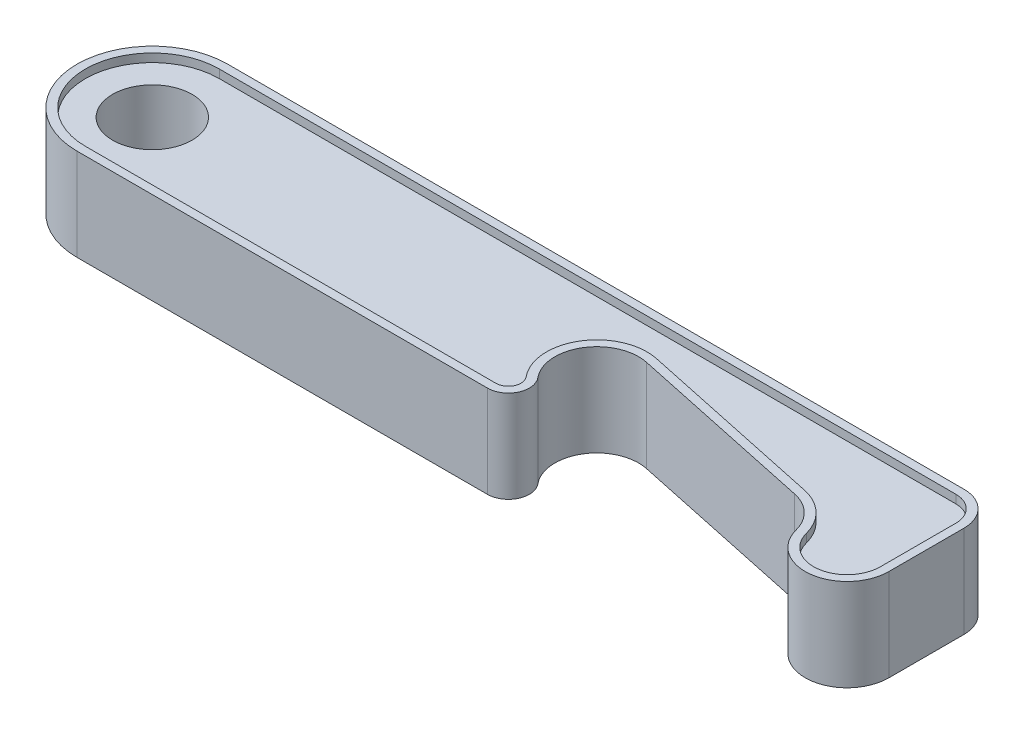
ISO-10303-21;
HEADER;
FILE_DESCRIPTION(('STEP AP214'),'2;1');
FILE_NAME('part.step','',(''),(''),'','','');
FILE_SCHEMA(('AUTOMOTIVE_DESIGN { 1 0 10303 214 1 1 1 1 }'));
ENDSEC;
DATA;
#1=APPLICATION_CONTEXT('core data for automotive mechanical design processes');
#2=APPLICATION_PROTOCOL_DEFINITION('international standard','automotive_design',2000,#1);
#3=PRODUCT_CONTEXT('',#1,'mechanical');
#4=PRODUCT('Part','Part','',(#3));
#5=PRODUCT_RELATED_PRODUCT_CATEGORY('part','',(#4));
#6=PRODUCT_DEFINITION_FORMATION('','',#4);
#7=PRODUCT_DEFINITION_CONTEXT('part definition',#1,'design');
#8=PRODUCT_DEFINITION('design','',#6,#7);
#9=PRODUCT_DEFINITION_SHAPE('','',#8);
#10=(LENGTH_UNIT() NAMED_UNIT(*) SI_UNIT(.MILLI.,.METRE.));
#11=(NAMED_UNIT(*) PLANE_ANGLE_UNIT() SI_UNIT($,.RADIAN.));
#12=(NAMED_UNIT(*) SI_UNIT($,.STERADIAN.) SOLID_ANGLE_UNIT());
#13=UNCERTAINTY_MEASURE_WITH_UNIT(LENGTH_MEASURE(1.E-05),#10,'distance_accuracy_value','');
#14=(GEOMETRIC_REPRESENTATION_CONTEXT(3) GLOBAL_UNCERTAINTY_ASSIGNED_CONTEXT((#13)) GLOBAL_UNIT_ASSIGNED_CONTEXT((#10,
#11,#12)) REPRESENTATION_CONTEXT('',''));
#15=CARTESIAN_POINT('',(0.,0.,0.));
#16=DIRECTION('',(0.,0.,1.));
#17=DIRECTION('',(1.,0.,0.));
#18=AXIS2_PLACEMENT_3D('',#15,#16,#17);
#19=CARTESIAN_POINT('',(-41.5,5.5,0.));
#20=DIRECTION('',(0.,-1.,0.));
#21=DIRECTION('',(0.,0.,-1.));
#22=AXIS2_PLACEMENT_3D('',#19,#20,#21);
#23=CYLINDRICAL_SURFACE('',#22,4.75);
#24=CARTESIAN_POINT('',(-41.5,4.5,0.));
#25=DIRECTION('',(0.,1.,0.));
#26=DIRECTION('',(0.,0.,1.));
#27=AXIS2_PLACEMENT_3D('',#24,#25,#26);
#28=CIRCLE('',#27,4.75);
#29=CARTESIAN_POINT('',(-41.5,4.5,4.75));
#30=VERTEX_POINT('',#29);
#31=EDGE_CURVE('E379',#30,#30,#28,.T.);
#32=ORIENTED_EDGE('',*,*,#31,.T.);
#33=EDGE_LOOP('',(#32));
#34=FACE_BOUND('',#33,.T.);
#35=CARTESIAN_POINT('',(-41.5,-4.5,0.));
#36=DIRECTION('',(0.,-1.,0.));
#37=DIRECTION('',(0.,0.,-1.));
#38=AXIS2_PLACEMENT_3D('',#35,#36,#37);
#39=CIRCLE('',#38,4.75);
#40=CARTESIAN_POINT('',(-41.5,-4.5,-4.74999999999999));
#41=VERTEX_POINT('',#40);
#42=EDGE_CURVE('E43',#41,#41,#39,.T.);
#43=ORIENTED_EDGE('',*,*,#42,.T.);
#44=EDGE_LOOP('',(#43));
#45=FACE_BOUND('',#44,.T.);
#46=ADVANCED_FACE('F39',(#34,#45),#23,.F.);
#47=CARTESIAN_POINT('',(-41.5,-5.5,0.));
#48=DIRECTION('',(0.,1.,0.));
#49=DIRECTION('',(0.,0.,1.));
#50=AXIS2_PLACEMENT_3D('',#47,#48,#49);
#51=PLANE('',#50);
#52=CARTESIAN_POINT('',(-41.5,-5.5,0.));
#53=DIRECTION('',(0.,1.,0.));
#54=DIRECTION('',(0.,0.,1.));
#55=AXIS2_PLACEMENT_3D('',#52,#53,#54);
#56=CIRCLE('',#55,9.);
#57=CARTESIAN_POINT('',(-41.5,-5.5,-8.99999999999999));
#58=VERTEX_POINT('',#57);
#59=CARTESIAN_POINT('',(-41.5,-5.5,9.00000000000001));
#60=VERTEX_POINT('',#59);
#61=EDGE_CURVE('E423',#58,#60,#56,.T.);
#62=ORIENTED_EDGE('',*,*,#61,.F.);
#63=DIRECTION('',(-1.,0.,0.));
#64=VECTOR('',#63,1.);
#65=CARTESIAN_POINT('',(46.5,-5.5,-9.));
#66=LINE('',#65,#64);
#67=CARTESIAN_POINT('',(46.5,-5.5,-9.));
#68=VERTEX_POINT('',#67);
#69=EDGE_CURVE('E405',#68,#58,#66,.T.);
#70=ORIENTED_EDGE('',*,*,#69,.F.);
#71=CARTESIAN_POINT('',(46.5,-5.5,-5.));
#72=DIRECTION('',(0.,1.,0.));
#73=DIRECTION('',(0.,0.,-1.));
#74=AXIS2_PLACEMENT_3D('',#71,#72,#73);
#75=CIRCLE('',#74,4.);
#76=CARTESIAN_POINT('',(50.5,-5.5,-4.99999999999998));
#77=VERTEX_POINT('',#76);
#78=EDGE_CURVE('E437',#77,#68,#75,.T.);
#79=ORIENTED_EDGE('',*,*,#78,.F.);
#80=DIRECTION('',(0.,0.,-1.));
#81=VECTOR('',#80,1.);
#82=CARTESIAN_POINT('',(50.5,-5.5,-4.99999999999997));
#83=LINE('',#82,#81);
#84=CARTESIAN_POINT('',(50.5,-5.5,3.99999999999999));
#85=VERTEX_POINT('',#84);
#86=EDGE_CURVE('E436',#85,#77,#83,.T.);
#87=ORIENTED_EDGE('',*,*,#86,.F.);
#88=CARTESIAN_POINT('',(45.5,-5.5,3.99999999999999));
#89=DIRECTION('',(0.,1.,0.));
#90=DIRECTION('',(0.,0.,1.));
#91=AXIS2_PLACEMENT_3D('',#88,#89,#90);
#92=CIRCLE('',#91,5.);
#93=CARTESIAN_POINT('',(40.6587708172407,-5.5,5.24999999999999));
#94=VERTEX_POINT('',#93);
#95=EDGE_CURVE('E432',#94,#85,#92,.T.);
#96=ORIENTED_EDGE('',*,*,#95,.F.);
#97=CARTESIAN_POINT('',(35.8175416344815,-5.5,6.49999999999999));
#98=DIRECTION('',(0.,-1.,0.));
#99=DIRECTION('',(0.,0.,1.));
#100=AXIS2_PLACEMENT_3D('',#97,#98,#99);
#101=CIRCLE('',#100,5.00000000000001);
#102=CARTESIAN_POINT('',(36.8571000885702,-5.5,1.60926199633095));
#103=VERTEX_POINT('',#102);
#104=EDGE_CURVE('E435',#103,#94,#101,.T.);
#105=ORIENTED_EDGE('',*,*,#104,.F.);
#106=DIRECTION('',(0.978147600733807,0.,0.207911690817752));
#107=VECTOR('',#106,1.);
#108=CARTESIAN_POINT('',(14.3571000885702,-5.5,-3.17326064124438));
#109=LINE('',#108,#107);
#110=CARTESIAN_POINT('',(14.3571000885702,-5.5,-3.17326064124438));
#111=VERTEX_POINT('',#110);
#112=EDGE_CURVE('E429',#111,#103,#109,.T.);
#113=ORIENTED_EDGE('',*,*,#112,.F.);
#114=CARTESIAN_POINT('',(13.3175416344815,-5.5,1.71747736242465));
#115=DIRECTION('',(0.,-1.,0.));
#116=DIRECTION('',(0.,0.,1.));
#117=AXIS2_PLACEMENT_3D('',#114,#115,#116);
#118=CIRCLE('',#117,5.);
#119=CARTESIAN_POINT('',(9.46599203458277,-5.5,4.90582578747488));
#120=VERTEX_POINT('',#119);
#121=EDGE_CURVE('E428',#120,#111,#118,.T.);
#122=ORIENTED_EDGE('',*,*,#121,.F.);
#123=CARTESIAN_POINT('',(7.54021723463343,-5.5,6.49999999999999));
#124=DIRECTION('',(0.,1.,0.));
#125=DIRECTION('',(0.,0.,1.));
#126=AXIS2_PLACEMENT_3D('',#123,#124,#125);
#127=CIRCLE('',#126,2.50000000000001);
#128=CARTESIAN_POINT('',(7.54021723463343,-5.5,8.99999999999999));
#129=VERTEX_POINT('',#128);
#130=EDGE_CURVE('E426',#129,#120,#127,.T.);
#131=ORIENTED_EDGE('',*,*,#130,.F.);
#132=DIRECTION('',(1.,0.,0.));
#133=VECTOR('',#132,1.);
#134=CARTESIAN_POINT('',(7.54021723463343,-5.5,9.));
#135=LINE('',#134,#133);
#136=EDGE_CURVE('E424',#60,#129,#135,.T.);
#137=ORIENTED_EDGE('',*,*,#136,.F.);
#138=EDGE_LOOP('',(#62,#70,#79,#87,#96,#105,#113,#122,#131,#137));
#139=FACE_BOUND('',#138,.T.);
#140=CARTESIAN_POINT('',(-41.5,-5.5,0.));
#141=DIRECTION('',(0.,1.,0.));
#142=DIRECTION('',(0.,0.,1.));
#143=AXIS2_PLACEMENT_3D('',#140,#141,#142);
#144=CIRCLE('',#143,8.);
#145=CARTESIAN_POINT('',(-41.5,-5.5,-7.99999999999999));
#146=VERTEX_POINT('',#145);
#147=CARTESIAN_POINT('',(-41.5,-5.5,8.));
#148=VERTEX_POINT('',#147);
#149=EDGE_CURVE('E57',#146,#148,#144,.T.);
#150=ORIENTED_EDGE('',*,*,#149,.T.);
#151=DIRECTION('',(1.,0.,0.));
#152=VECTOR('',#151,1.);
#153=CARTESIAN_POINT('',(-41.5,-5.5,8.));
#154=LINE('',#153,#152);
#155=CARTESIAN_POINT('',(7.54021723463342,-5.5,7.99999999999999));
#156=VERTEX_POINT('',#155);
#157=EDGE_CURVE('E259',#148,#156,#154,.T.);
#158=ORIENTED_EDGE('',*,*,#157,.T.);
#159=CARTESIAN_POINT('',(7.54021723463343,-5.5,6.49999999999999));
#160=DIRECTION('',(0.,1.,0.));
#161=DIRECTION('',(0.,0.,1.));
#162=AXIS2_PLACEMENT_3D('',#159,#160,#161);
#163=CIRCLE('',#162,1.5);
#164=CARTESIAN_POINT('',(8.69568211460303,-5.5,5.54349547248492));
#165=VERTEX_POINT('',#164);
#166=EDGE_CURVE('E265',#156,#165,#163,.T.);
#167=ORIENTED_EDGE('',*,*,#166,.T.);
#168=CARTESIAN_POINT('',(13.3175416344815,-5.5,1.71747736242465));
#169=DIRECTION('',(0.,-1.,0.));
#170=DIRECTION('',(0.,0.,1.));
#171=AXIS2_PLACEMENT_3D('',#168,#169,#170);
#172=CIRCLE('',#171,6.);
#173=CARTESIAN_POINT('',(14.565011779388,-5.5,-4.15140824197819));
#174=VERTEX_POINT('',#173);
#175=EDGE_CURVE('E300',#165,#174,#172,.T.);
#176=ORIENTED_EDGE('',*,*,#175,.T.);
#177=DIRECTION('',(0.978147600733807,0.,0.207911690817753));
#178=VECTOR('',#177,1.);
#179=CARTESIAN_POINT('',(14.565011779388,-5.5,-4.15140824197819));
#180=LINE('',#179,#178);
#181=CARTESIAN_POINT('',(37.065011779388,-5.5,0.631114395597146));
#182=VERTEX_POINT('',#181);
#183=EDGE_CURVE('E294',#174,#182,#180,.T.);
#184=ORIENTED_EDGE('',*,*,#183,.T.);
#185=CARTESIAN_POINT('',(35.8175416344815,-5.5,6.49999999999999));
#186=DIRECTION('',(0.,-1.,0.));
#187=DIRECTION('',(0.,0.,1.));
#188=AXIS2_PLACEMENT_3D('',#185,#186,#187);
#189=CIRCLE('',#188,6.00000000000001);
#190=CARTESIAN_POINT('',(41.6270166537926,-5.5,4.99999999999999));
#191=VERTEX_POINT('',#190);
#192=EDGE_CURVE('E292',#182,#191,#189,.T.);
#193=ORIENTED_EDGE('',*,*,#192,.T.);
#194=CARTESIAN_POINT('',(45.5,-5.5,3.99999999999999));
#195=DIRECTION('',(0.,1.,0.));
#196=DIRECTION('',(0.,0.,1.));
#197=AXIS2_PLACEMENT_3D('',#194,#195,#196);
#198=CIRCLE('',#197,4.);
#199=CARTESIAN_POINT('',(49.5,-5.5,3.99999999999999));
#200=VERTEX_POINT('',#199);
#201=EDGE_CURVE('E290',#191,#200,#198,.T.);
#202=ORIENTED_EDGE('',*,*,#201,.T.);
#203=DIRECTION('',(0.,0.,-1.));
#204=VECTOR('',#203,1.);
#205=CARTESIAN_POINT('',(49.5,-5.5,3.99999999999999));
#206=LINE('',#205,#204);
#207=CARTESIAN_POINT('',(49.5,-5.5,-4.99999999999998));
#208=VERTEX_POINT('',#207);
#209=EDGE_CURVE('E284',#200,#208,#206,.T.);
#210=ORIENTED_EDGE('',*,*,#209,.T.);
#211=CARTESIAN_POINT('',(46.5,-5.5,-5.));
#212=DIRECTION('',(0.,1.,0.));
#213=DIRECTION('',(0.,0.,1.));
#214=AXIS2_PLACEMENT_3D('',#211,#212,#213);
#215=CIRCLE('',#214,3.);
#216=CARTESIAN_POINT('',(46.5,-5.5,-8.));
#217=VERTEX_POINT('',#216);
#218=EDGE_CURVE('E285',#208,#217,#215,.T.);
#219=ORIENTED_EDGE('',*,*,#218,.T.);
#220=DIRECTION('',(-1.,0.,0.));
#221=VECTOR('',#220,1.);
#222=CARTESIAN_POINT('',(46.5,-5.5,-8.));
#223=LINE('',#222,#221);
#224=EDGE_CURVE('E278',#217,#146,#223,.T.);
#225=ORIENTED_EDGE('',*,*,#224,.T.);
#226=EDGE_LOOP('',(#150,#158,#167,#176,#184,#193,#202,#210,#219,#225));
#227=FACE_BOUND('',#226,.T.);
#228=ADVANCED_FACE('F516',(#139,#227),#51,.F.);
#229=CARTESIAN_POINT('',(-41.5,5.5,0.));
#230=DIRECTION('',(0.,1.,0.));
#231=DIRECTION('',(0.,0.,1.));
#232=AXIS2_PLACEMENT_3D('',#229,#230,#231);
#233=PLANE('',#232);
#234=CARTESIAN_POINT('',(-41.5,5.5,0.));
#235=DIRECTION('',(0.,1.,0.));
#236=DIRECTION('',(0.,0.,1.));
#237=AXIS2_PLACEMENT_3D('',#234,#235,#236);
#238=CIRCLE('',#237,8.);
#239=CARTESIAN_POINT('',(-41.5,5.5,-7.99999999999999));
#240=VERTEX_POINT('',#239);
#241=CARTESIAN_POINT('',(-41.5,5.5,8.));
#242=VERTEX_POINT('',#241);
#243=EDGE_CURVE('E63',#240,#242,#238,.T.);
#244=ORIENTED_EDGE('',*,*,#243,.F.);
#245=DIRECTION('',(-1.,0.,0.));
#246=VECTOR('',#245,1.);
#247=CARTESIAN_POINT('',(46.5,5.5,-8.));
#248=LINE('',#247,#246);
#249=CARTESIAN_POINT('',(46.5,5.5,-8.));
#250=VERTEX_POINT('',#249);
#251=EDGE_CURVE('E323',#250,#240,#248,.T.);
#252=ORIENTED_EDGE('',*,*,#251,.F.);
#253=CARTESIAN_POINT('',(46.5,5.5,-5.));
#254=DIRECTION('',(0.,1.,0.));
#255=DIRECTION('',(0.,0.,1.));
#256=AXIS2_PLACEMENT_3D('',#253,#254,#255);
#257=CIRCLE('',#256,3.);
#258=CARTESIAN_POINT('',(49.5,5.5,-4.99999999999998));
#259=VERTEX_POINT('',#258);
#260=EDGE_CURVE('E373',#259,#250,#257,.T.);
#261=ORIENTED_EDGE('',*,*,#260,.F.);
#262=DIRECTION('',(0.,0.,-1.));
#263=VECTOR('',#262,1.);
#264=CARTESIAN_POINT('',(49.5,5.5,3.99999999999999));
#265=LINE('',#264,#263);
#266=CARTESIAN_POINT('',(49.5,5.5,3.99999999999999));
#267=VERTEX_POINT('',#266);
#268=EDGE_CURVE('E367',#267,#259,#265,.T.);
#269=ORIENTED_EDGE('',*,*,#268,.F.);
#270=CARTESIAN_POINT('',(45.5,5.5,3.99999999999999));
#271=DIRECTION('',(0.,1.,0.));
#272=DIRECTION('',(0.,0.,1.));
#273=AXIS2_PLACEMENT_3D('',#270,#271,#272);
#274=CIRCLE('',#273,4.);
#275=CARTESIAN_POINT('',(41.6270166537926,5.5,4.99999999999999));
#276=VERTEX_POINT('',#275);
#277=EDGE_CURVE('E370',#276,#267,#274,.T.);
#278=ORIENTED_EDGE('',*,*,#277,.F.);
#279=CARTESIAN_POINT('',(35.8175416344815,5.5,6.49999999999999));
#280=DIRECTION('',(0.,-1.,0.));
#281=DIRECTION('',(0.,0.,1.));
#282=AXIS2_PLACEMENT_3D('',#279,#280,#281);
#283=CIRCLE('',#282,6.00000000000001);
#284=CARTESIAN_POINT('',(37.065011779388,5.5,0.631114395597146));
#285=VERTEX_POINT('',#284);
#286=EDGE_CURVE('E365',#285,#276,#283,.T.);
#287=ORIENTED_EDGE('',*,*,#286,.F.);
#288=DIRECTION('',(0.978147600733807,0.,0.207911690817753));
#289=VECTOR('',#288,1.);
#290=CARTESIAN_POINT('',(14.565011779388,5.5,-4.15140824197819));
#291=LINE('',#290,#289);
#292=CARTESIAN_POINT('',(14.565011779388,5.5,-4.15140824197819));
#293=VERTEX_POINT('',#292);
#294=EDGE_CURVE('E363',#293,#285,#291,.T.);
#295=ORIENTED_EDGE('',*,*,#294,.F.);
#296=CARTESIAN_POINT('',(13.3175416344815,5.5,1.71747736242465));
#297=DIRECTION('',(0.,-1.,0.));
#298=DIRECTION('',(0.,0.,1.));
#299=AXIS2_PLACEMENT_3D('',#296,#297,#298);
#300=CIRCLE('',#299,6.);
#301=CARTESIAN_POINT('',(8.69568211460303,5.5,5.54349547248492));
#302=VERTEX_POINT('',#301);
#303=EDGE_CURVE('E360',#302,#293,#300,.T.);
#304=ORIENTED_EDGE('',*,*,#303,.F.);
#305=CARTESIAN_POINT('',(7.54021723463343,5.5,6.49999999999999));
#306=DIRECTION('',(0.,1.,0.));
#307=DIRECTION('',(0.,0.,1.));
#308=AXIS2_PLACEMENT_3D('',#305,#306,#307);
#309=CIRCLE('',#308,1.5);
#310=CARTESIAN_POINT('',(7.54021723463342,5.5,7.99999999999999));
#311=VERTEX_POINT('',#310);
#312=EDGE_CURVE('E354',#311,#302,#309,.T.);
#313=ORIENTED_EDGE('',*,*,#312,.F.);
#314=DIRECTION('',(1.,0.,0.));
#315=VECTOR('',#314,1.);
#316=CARTESIAN_POINT('',(-41.5,5.5,8.));
#317=LINE('',#316,#315);
#318=EDGE_CURVE('E355',#242,#311,#317,.T.);
#319=ORIENTED_EDGE('',*,*,#318,.F.);
#320=EDGE_LOOP('',(#244,#252,#261,#269,#278,#287,#295,#304,#313,#319));
#321=FACE_BOUND('',#320,.T.);
#322=CARTESIAN_POINT('',(-41.5,5.5,0.));
#323=DIRECTION('',(0.,1.,0.));
#324=DIRECTION('',(0.,0.,1.));
#325=AXIS2_PLACEMENT_3D('',#322,#323,#324);
#326=CIRCLE('',#325,9.);
#327=CARTESIAN_POINT('',(-41.5,5.5,-8.99999999999999));
#328=VERTEX_POINT('',#327);
#329=CARTESIAN_POINT('',(-41.5,5.5,9.00000000000001));
#330=VERTEX_POINT('',#329);
#331=EDGE_CURVE('E400',#328,#330,#326,.T.);
#332=ORIENTED_EDGE('',*,*,#331,.T.);
#333=DIRECTION('',(1.,0.,0.));
#334=VECTOR('',#333,1.);
#335=CARTESIAN_POINT('',(7.54021723463343,5.5,9.));
#336=LINE('',#335,#334);
#337=CARTESIAN_POINT('',(7.54021723463343,5.5,8.99999999999999));
#338=VERTEX_POINT('',#337);
#339=EDGE_CURVE('E402',#330,#338,#336,.T.);
#340=ORIENTED_EDGE('',*,*,#339,.T.);
#341=CARTESIAN_POINT('',(7.54021723463343,5.5,6.49999999999999));
#342=DIRECTION('',(0.,1.,0.));
#343=DIRECTION('',(0.,0.,1.));
#344=AXIS2_PLACEMENT_3D('',#341,#342,#343);
#345=CIRCLE('',#344,2.50000000000001);
#346=CARTESIAN_POINT('',(9.46599203458277,5.5,4.90582578747488));
#347=VERTEX_POINT('',#346);
#348=EDGE_CURVE('E404',#338,#347,#345,.T.);
#349=ORIENTED_EDGE('',*,*,#348,.T.);
#350=CARTESIAN_POINT('',(13.3175416344815,5.5,1.71747736242465));
#351=DIRECTION('',(0.,-1.,0.));
#352=DIRECTION('',(0.,0.,1.));
#353=AXIS2_PLACEMENT_3D('',#350,#351,#352);
#354=CIRCLE('',#353,5.);
#355=CARTESIAN_POINT('',(14.3571000885702,5.5,-3.17326064124438));
#356=VERTEX_POINT('',#355);
#357=EDGE_CURVE('E406',#347,#356,#354,.T.);
#358=ORIENTED_EDGE('',*,*,#357,.T.);
#359=DIRECTION('',(0.978147600733807,0.,0.207911690817752));
#360=VECTOR('',#359,1.);
#361=CARTESIAN_POINT('',(14.3571000885702,5.5,-3.17326064124438));
#362=LINE('',#361,#360);
#363=CARTESIAN_POINT('',(36.8571000885702,5.5,1.60926199633095));
#364=VERTEX_POINT('',#363);
#365=EDGE_CURVE('E407',#356,#364,#362,.T.);
#366=ORIENTED_EDGE('',*,*,#365,.T.);
#367=CARTESIAN_POINT('',(35.8175416344815,5.5,6.49999999999999));
#368=DIRECTION('',(0.,-1.,0.));
#369=DIRECTION('',(0.,0.,1.));
#370=AXIS2_PLACEMENT_3D('',#367,#368,#369);
#371=CIRCLE('',#370,5.00000000000001);
#372=CARTESIAN_POINT('',(40.6587708172407,5.5,5.24999999999999));
#373=VERTEX_POINT('',#372);
#374=EDGE_CURVE('E409',#364,#373,#371,.T.);
#375=ORIENTED_EDGE('',*,*,#374,.T.);
#376=CARTESIAN_POINT('',(45.5,5.5,3.99999999999999));
#377=DIRECTION('',(0.,1.,0.));
#378=DIRECTION('',(0.,0.,1.));
#379=AXIS2_PLACEMENT_3D('',#376,#377,#378);
#380=CIRCLE('',#379,5.);
#381=CARTESIAN_POINT('',(50.5,5.5,3.99999999999999));
#382=VERTEX_POINT('',#381);
#383=EDGE_CURVE('E411',#373,#382,#380,.T.);
#384=ORIENTED_EDGE('',*,*,#383,.T.);
#385=DIRECTION('',(0.,0.,-1.));
#386=VECTOR('',#385,1.);
#387=CARTESIAN_POINT('',(50.5,5.5,-4.99999999999997));
#388=LINE('',#387,#386);
#389=CARTESIAN_POINT('',(50.5,5.5,-4.99999999999998));
#390=VERTEX_POINT('',#389);
#391=EDGE_CURVE('E413',#382,#390,#388,.T.);
#392=ORIENTED_EDGE('',*,*,#391,.T.);
#393=CARTESIAN_POINT('',(46.5,5.5,-5.));
#394=DIRECTION('',(0.,1.,0.));
#395=DIRECTION('',(0.,0.,-1.));
#396=AXIS2_PLACEMENT_3D('',#393,#394,#395);
#397=CIRCLE('',#396,4.);
#398=CARTESIAN_POINT('',(46.5,5.5,-9.));
#399=VERTEX_POINT('',#398);
#400=EDGE_CURVE('E418',#390,#399,#397,.T.);
#401=ORIENTED_EDGE('',*,*,#400,.T.);
#402=DIRECTION('',(-1.,0.,0.));
#403=VECTOR('',#402,1.);
#404=CARTESIAN_POINT('',(46.5,5.5,-9.));
#405=LINE('',#404,#403);
#406=EDGE_CURVE('E416',#399,#328,#405,.T.);
#407=ORIENTED_EDGE('',*,*,#406,.T.);
#408=EDGE_LOOP('',(#332,#340,#349,#358,#366,#375,#384,#392,#401,#407));
#409=FACE_BOUND('',#408,.T.);
#410=ADVANCED_FACE('F511',(#321,#409),#233,.T.);
#411=CARTESIAN_POINT('',(-41.5,5.5,0.));
#412=DIRECTION('',(0.,-1.,0.));
#413=DIRECTION('',(0.,0.,-1.));
#414=AXIS2_PLACEMENT_3D('',#411,#412,#413);
#415=CYLINDRICAL_SURFACE('',#414,9.);
#416=ORIENTED_EDGE('',*,*,#61,.T.);
#417=DIRECTION('',(0.,-1.,0.));
#418=VECTOR('',#417,1.);
#419=CARTESIAN_POINT('',(-41.5,5.5,9.00000000000001));
#420=LINE('',#419,#418);
#421=EDGE_CURVE('E11',#330,#60,#420,.T.);
#422=ORIENTED_EDGE('',*,*,#421,.F.);
#423=ORIENTED_EDGE('',*,*,#331,.F.);
#424=DIRECTION('',(0.,-1.,0.));
#425=VECTOR('',#424,1.);
#426=CARTESIAN_POINT('',(-41.5,5.5,-8.99999999999999));
#427=LINE('',#426,#425);
#428=EDGE_CURVE('E419',#328,#58,#427,.T.);
#429=ORIENTED_EDGE('',*,*,#428,.T.);
#430=EDGE_LOOP('',(#416,#422,#423,#429));
#431=FACE_BOUND('',#430,.T.);
#432=ADVANCED_FACE('F41',(#431),#415,.T.);
#433=CARTESIAN_POINT('',(7.54021723463343,5.5,9.));
#434=DIRECTION('',(0.,0.,-1.));
#435=DIRECTION('',(-1.,0.,0.));
#436=AXIS2_PLACEMENT_3D('',#433,#434,#435);
#437=PLANE('',#436);
#438=ORIENTED_EDGE('',*,*,#136,.T.);
#439=DIRECTION('',(0.,-1.,0.));
#440=VECTOR('',#439,1.);
#441=CARTESIAN_POINT('',(7.54021723463343,5.5,8.99999999999999));
#442=LINE('',#441,#440);
#443=EDGE_CURVE('E48',#338,#129,#442,.T.);
#444=ORIENTED_EDGE('',*,*,#443,.F.);
#445=ORIENTED_EDGE('',*,*,#339,.F.);
#446=ORIENTED_EDGE('',*,*,#421,.T.);
#447=EDGE_LOOP('',(#438,#444,#445,#446));
#448=FACE_BOUND('',#447,.T.);
#449=ADVANCED_FACE('F528',(#448),#437,.F.);
#450=CARTESIAN_POINT('',(7.54021723463343,5.5,6.49999999999999));
#451=DIRECTION('',(0.,-1.,0.));
#452=DIRECTION('',(0.,0.,-1.));
#453=AXIS2_PLACEMENT_3D('',#450,#451,#452);
#454=CYLINDRICAL_SURFACE('',#453,2.50000000000001);
#455=ORIENTED_EDGE('',*,*,#130,.T.);
#456=DIRECTION('',(0.,-1.,0.));
#457=VECTOR('',#456,1.);
#458=CARTESIAN_POINT('',(9.46599203458277,5.5,4.90582578747488));
#459=LINE('',#458,#457);
#460=EDGE_CURVE('E461',#347,#120,#459,.T.);
#461=ORIENTED_EDGE('',*,*,#460,.F.);
#462=ORIENTED_EDGE('',*,*,#348,.F.);
#463=ORIENTED_EDGE('',*,*,#443,.T.);
#464=EDGE_LOOP('',(#455,#461,#462,#463));
#465=FACE_BOUND('',#464,.T.);
#466=ADVANCED_FACE('F533',(#465),#454,.T.);
#467=CARTESIAN_POINT('',(13.3175416344815,5.5,1.71747736242465));
#468=DIRECTION('',(0.,-1.,0.));
#469=DIRECTION('',(0.,0.,-1.));
#470=AXIS2_PLACEMENT_3D('',#467,#468,#469);
#471=CYLINDRICAL_SURFACE('',#470,5.);
#472=ORIENTED_EDGE('',*,*,#121,.T.);
#473=DIRECTION('',(0.,-1.,0.));
#474=VECTOR('',#473,1.);
#475=CARTESIAN_POINT('',(14.3571000885702,5.5,-3.17326064124438));
#476=LINE('',#475,#474);
#477=EDGE_CURVE('E456',#356,#111,#476,.T.);
#478=ORIENTED_EDGE('',*,*,#477,.F.);
#479=ORIENTED_EDGE('',*,*,#357,.F.);
#480=ORIENTED_EDGE('',*,*,#460,.T.);
#481=EDGE_LOOP('',(#472,#478,#479,#480));
#482=FACE_BOUND('',#481,.T.);
#483=ADVANCED_FACE('F540',(#482),#471,.F.);
#484=CARTESIAN_POINT('',(14.3571000885702,5.5,-3.17326064124438));
#485=DIRECTION('',(0.207911690817752,0.,-0.978147600733807));
#486=DIRECTION('',(-0.978147600733807,0.,-0.207911690817752));
#487=AXIS2_PLACEMENT_3D('',#484,#485,#486);
#488=PLANE('',#487);
#489=ORIENTED_EDGE('',*,*,#112,.T.);
#490=DIRECTION('',(0.,-1.,0.));
#491=VECTOR('',#490,1.);
#492=CARTESIAN_POINT('',(36.8571000885702,5.5,1.60926199633095));
#493=LINE('',#492,#491);
#494=EDGE_CURVE('E452',#364,#103,#493,.T.);
#495=ORIENTED_EDGE('',*,*,#494,.F.);
#496=ORIENTED_EDGE('',*,*,#365,.F.);
#497=ORIENTED_EDGE('',*,*,#477,.T.);
#498=EDGE_LOOP('',(#489,#495,#496,#497));
#499=FACE_BOUND('',#498,.T.);
#500=ADVANCED_FACE('F541',(#499),#488,.F.);
#501=CARTESIAN_POINT('',(35.8175416344815,5.5,6.49999999999999));
#502=DIRECTION('',(0.,-1.,0.));
#503=DIRECTION('',(0.,0.,-1.));
#504=AXIS2_PLACEMENT_3D('',#501,#502,#503);
#505=CYLINDRICAL_SURFACE('',#504,5.00000000000001);
#506=ORIENTED_EDGE('',*,*,#104,.T.);
#507=DIRECTION('',(0.,-1.,0.));
#508=VECTOR('',#507,1.);
#509=CARTESIAN_POINT('',(40.6587708172407,5.5,5.24999999999999));
#510=LINE('',#509,#508);
#511=EDGE_CURVE('E451',#373,#94,#510,.T.);
#512=ORIENTED_EDGE('',*,*,#511,.F.);
#513=ORIENTED_EDGE('',*,*,#374,.F.);
#514=ORIENTED_EDGE('',*,*,#494,.T.);
#515=EDGE_LOOP('',(#506,#512,#513,#514));
#516=FACE_BOUND('',#515,.T.);
#517=ADVANCED_FACE('F546',(#516),#505,.F.);
#518=CARTESIAN_POINT('',(45.5,5.5,3.99999999999999));
#519=DIRECTION('',(0.,-1.,0.));
#520=DIRECTION('',(0.,0.,-1.));
#521=AXIS2_PLACEMENT_3D('',#518,#519,#520);
#522=CYLINDRICAL_SURFACE('',#521,5.);
#523=ORIENTED_EDGE('',*,*,#95,.T.);
#524=DIRECTION('',(0.,-1.,0.));
#525=VECTOR('',#524,1.);
#526=CARTESIAN_POINT('',(50.5,5.5,3.99999999999999));
#527=LINE('',#526,#525);
#528=EDGE_CURVE('E448',#382,#85,#527,.T.);
#529=ORIENTED_EDGE('',*,*,#528,.F.);
#530=ORIENTED_EDGE('',*,*,#383,.F.);
#531=ORIENTED_EDGE('',*,*,#511,.T.);
#532=EDGE_LOOP('',(#523,#529,#530,#531));
#533=FACE_BOUND('',#532,.T.);
#534=ADVANCED_FACE('F555',(#533),#522,.T.);
#535=CARTESIAN_POINT('',(50.5,5.5,-4.99999999999997));
#536=DIRECTION('',(-1.,0.,0.));
#537=DIRECTION('',(0.,0.,1.));
#538=AXIS2_PLACEMENT_3D('',#535,#536,#537);
#539=PLANE('',#538);
#540=ORIENTED_EDGE('',*,*,#86,.T.);
#541=DIRECTION('',(0.,-1.,0.));
#542=VECTOR('',#541,1.);
#543=CARTESIAN_POINT('',(50.5,5.5,-4.99999999999998));
#544=LINE('',#543,#542);
#545=EDGE_CURVE('E446',#390,#77,#544,.T.);
#546=ORIENTED_EDGE('',*,*,#545,.F.);
#547=ORIENTED_EDGE('',*,*,#391,.F.);
#548=ORIENTED_EDGE('',*,*,#528,.T.);
#549=EDGE_LOOP('',(#540,#546,#547,#548));
#550=FACE_BOUND('',#549,.T.);
#551=ADVANCED_FACE('F556',(#550),#539,.F.);
#552=CARTESIAN_POINT('',(46.5,5.5,-5.));
#553=DIRECTION('',(0.,-1.,0.));
#554=DIRECTION('',(0.,0.,-1.));
#555=AXIS2_PLACEMENT_3D('',#552,#553,#554);
#556=CYLINDRICAL_SURFACE('',#555,4.);
#557=ORIENTED_EDGE('',*,*,#78,.T.);
#558=DIRECTION('',(0.,-1.,0.));
#559=VECTOR('',#558,1.);
#560=CARTESIAN_POINT('',(46.5,5.5,-9.));
#561=LINE('',#560,#559);
#562=EDGE_CURVE('E444',#399,#68,#561,.T.);
#563=ORIENTED_EDGE('',*,*,#562,.F.);
#564=ORIENTED_EDGE('',*,*,#400,.F.);
#565=ORIENTED_EDGE('',*,*,#545,.T.);
#566=EDGE_LOOP('',(#557,#563,#564,#565));
#567=FACE_BOUND('',#566,.T.);
#568=ADVANCED_FACE('F564',(#567),#556,.T.);
#569=CARTESIAN_POINT('',(46.5,5.5,-9.));
#570=DIRECTION('',(0.,0.,1.));
#571=DIRECTION('',(1.,0.,0.));
#572=AXIS2_PLACEMENT_3D('',#569,#570,#571);
#573=PLANE('',#572);
#574=ORIENTED_EDGE('',*,*,#69,.T.);
#575=ORIENTED_EDGE('',*,*,#428,.F.);
#576=ORIENTED_EDGE('',*,*,#406,.F.);
#577=ORIENTED_EDGE('',*,*,#562,.T.);
#578=EDGE_LOOP('',(#574,#575,#576,#577));
#579=FACE_BOUND('',#578,.T.);
#580=ADVANCED_FACE('F563',(#579),#573,.F.);
#581=CARTESIAN_POINT('',(-41.5,4.5,0.));
#582=DIRECTION('',(0.,1.,0.));
#583=DIRECTION('',(0.,0.,1.));
#584=AXIS2_PLACEMENT_3D('',#581,#582,#583);
#585=CYLINDRICAL_SURFACE('',#584,8.);
#586=ORIENTED_EDGE('',*,*,#243,.T.);
#587=DIRECTION('',(0.,1.,0.));
#588=VECTOR('',#587,1.);
#589=CARTESIAN_POINT('',(-41.5,4.5,8.));
#590=LINE('',#589,#588);
#591=CARTESIAN_POINT('',(-41.5,4.5,8.));
#592=VERTEX_POINT('',#591);
#593=EDGE_CURVE('E348',#592,#242,#590,.T.);
#594=ORIENTED_EDGE('',*,*,#593,.F.);
#595=CARTESIAN_POINT('',(-41.5,4.5,0.));
#596=DIRECTION('',(0.,1.,0.));
#597=DIRECTION('',(0.,0.,1.));
#598=AXIS2_PLACEMENT_3D('',#595,#596,#597);
#599=CIRCLE('',#598,8.);
#600=CARTESIAN_POINT('',(-41.5,4.5,-7.99999999999999));
#601=VERTEX_POINT('',#600);
#602=EDGE_CURVE('E317',#601,#592,#599,.T.);
#603=ORIENTED_EDGE('',*,*,#602,.F.);
#604=DIRECTION('',(0.,1.,0.));
#605=VECTOR('',#604,1.);
#606=CARTESIAN_POINT('',(-41.5,4.5,-7.99999999999999));
#607=LINE('',#606,#605);
#608=EDGE_CURVE('E378',#601,#240,#607,.T.);
#609=ORIENTED_EDGE('',*,*,#608,.T.);
#610=EDGE_LOOP('',(#586,#594,#603,#609));
#611=FACE_BOUND('',#610,.T.);
#612=ADVANCED_FACE('F476',(#611),#585,.F.);
#613=CARTESIAN_POINT('',(46.5,4.5,-8.));
#614=DIRECTION('',(0.,0.,-1.));
#615=DIRECTION('',(-1.,0.,0.));
#616=AXIS2_PLACEMENT_3D('',#613,#614,#615);
#617=PLANE('',#616);
#618=ORIENTED_EDGE('',*,*,#251,.T.);
#619=ORIENTED_EDGE('',*,*,#608,.F.);
#620=DIRECTION('',(-1.,0.,0.));
#621=VECTOR('',#620,1.);
#622=CARTESIAN_POINT('',(46.5,4.5,-8.));
#623=LINE('',#622,#621);
#624=CARTESIAN_POINT('',(46.5,4.5,-8.));
#625=VERTEX_POINT('',#624);
#626=EDGE_CURVE('E350',#625,#601,#623,.T.);
#627=ORIENTED_EDGE('',*,*,#626,.F.);
#628=DIRECTION('',(0.,1.,0.));
#629=VECTOR('',#628,1.);
#630=CARTESIAN_POINT('',(46.5,4.5,-8.));
#631=LINE('',#630,#629);
#632=EDGE_CURVE('E381',#625,#250,#631,.T.);
#633=ORIENTED_EDGE('',*,*,#632,.T.);
#634=EDGE_LOOP('',(#618,#619,#627,#633));
#635=FACE_BOUND('',#634,.T.);
#636=ADVANCED_FACE('F507',(#635),#617,.F.);
#637=CARTESIAN_POINT('',(46.5,4.5,-5.));
#638=DIRECTION('',(0.,1.,0.));
#639=DIRECTION('',(0.,0.,1.));
#640=AXIS2_PLACEMENT_3D('',#637,#638,#639);
#641=CYLINDRICAL_SURFACE('',#640,3.);
#642=ORIENTED_EDGE('',*,*,#260,.T.);
#643=ORIENTED_EDGE('',*,*,#632,.F.);
#644=CARTESIAN_POINT('',(46.5,4.5,-5.));
#645=DIRECTION('',(0.,1.,0.));
#646=DIRECTION('',(0.,0.,1.));
#647=AXIS2_PLACEMENT_3D('',#644,#645,#646);
#648=CIRCLE('',#647,3.);
#649=CARTESIAN_POINT('',(49.5,4.5,-4.99999999999998));
#650=VERTEX_POINT('',#649);
#651=EDGE_CURVE('E343',#650,#625,#648,.T.);
#652=ORIENTED_EDGE('',*,*,#651,.F.);
#653=DIRECTION('',(0.,1.,0.));
#654=VECTOR('',#653,1.);
#655=CARTESIAN_POINT('',(49.5,4.5,-4.99999999999998));
#656=LINE('',#655,#654);
#657=EDGE_CURVE('E382',#650,#259,#656,.T.);
#658=ORIENTED_EDGE('',*,*,#657,.T.);
#659=EDGE_LOOP('',(#642,#643,#652,#658));
#660=FACE_BOUND('',#659,.T.);
#661=ADVANCED_FACE('F510',(#660),#641,.F.);
#662=CARTESIAN_POINT('',(49.5,4.5,3.99999999999999));
#663=DIRECTION('',(1.,0.,0.));
#664=DIRECTION('',(0.,0.,-1.));
#665=AXIS2_PLACEMENT_3D('',#662,#663,#664);
#666=PLANE('',#665);
#667=ORIENTED_EDGE('',*,*,#268,.T.);
#668=ORIENTED_EDGE('',*,*,#657,.F.);
#669=DIRECTION('',(0.,0.,-1.));
#670=VECTOR('',#669,1.);
#671=CARTESIAN_POINT('',(49.5,4.5,3.99999999999999));
#672=LINE('',#671,#670);
#673=CARTESIAN_POINT('',(49.5,4.5,3.99999999999999));
#674=VERTEX_POINT('',#673);
#675=EDGE_CURVE('E344',#674,#650,#672,.T.);
#676=ORIENTED_EDGE('',*,*,#675,.F.);
#677=DIRECTION('',(0.,1.,0.));
#678=VECTOR('',#677,1.);
#679=CARTESIAN_POINT('',(49.5,4.5,3.99999999999999));
#680=LINE('',#679,#678);
#681=EDGE_CURVE('E384',#674,#267,#680,.T.);
#682=ORIENTED_EDGE('',*,*,#681,.T.);
#683=EDGE_LOOP('',(#667,#668,#676,#682));
#684=FACE_BOUND('',#683,.T.);
#685=ADVANCED_FACE('F503',(#684),#666,.F.);
#686=CARTESIAN_POINT('',(45.5,4.5,3.99999999999999));
#687=DIRECTION('',(0.,1.,0.));
#688=DIRECTION('',(0.,0.,1.));
#689=AXIS2_PLACEMENT_3D('',#686,#687,#688);
#690=CYLINDRICAL_SURFACE('',#689,4.);
#691=ORIENTED_EDGE('',*,*,#277,.T.);
#692=ORIENTED_EDGE('',*,*,#681,.F.);
#693=CARTESIAN_POINT('',(45.5,4.5,3.99999999999999));
#694=DIRECTION('',(0.,1.,0.));
#695=DIRECTION('',(0.,0.,1.));
#696=AXIS2_PLACEMENT_3D('',#693,#694,#695);
#697=CIRCLE('',#696,4.);
#698=CARTESIAN_POINT('',(41.6270166537926,4.5,4.99999999999999));
#699=VERTEX_POINT('',#698);
#700=EDGE_CURVE('E337',#699,#674,#697,.T.);
#701=ORIENTED_EDGE('',*,*,#700,.F.);
#702=DIRECTION('',(0.,1.,0.));
#703=VECTOR('',#702,1.);
#704=CARTESIAN_POINT('',(41.6270166537926,4.5,4.99999999999999));
#705=LINE('',#704,#703);
#706=EDGE_CURVE('E390',#699,#276,#705,.T.);
#707=ORIENTED_EDGE('',*,*,#706,.T.);
#708=EDGE_LOOP('',(#691,#692,#701,#707));
#709=FACE_BOUND('',#708,.T.);
#710=ADVANCED_FACE('F498',(#709),#690,.F.);
#711=CARTESIAN_POINT('',(35.8175416344815,4.5,6.49999999999999));
#712=DIRECTION('',(0.,1.,0.));
#713=DIRECTION('',(0.,0.,1.));
#714=AXIS2_PLACEMENT_3D('',#711,#712,#713);
#715=CYLINDRICAL_SURFACE('',#714,6.00000000000001);
#716=ORIENTED_EDGE('',*,*,#286,.T.);
#717=ORIENTED_EDGE('',*,*,#706,.F.);
#718=CARTESIAN_POINT('',(35.8175416344815,4.5,6.49999999999999));
#719=DIRECTION('',(0.,-1.,0.));
#720=DIRECTION('',(0.,0.,1.));
#721=AXIS2_PLACEMENT_3D('',#718,#719,#720);
#722=CIRCLE('',#721,6.00000000000001);
#723=CARTESIAN_POINT('',(37.065011779388,4.5,0.631114395597146));
#724=VERTEX_POINT('',#723);
#725=EDGE_CURVE('E333',#724,#699,#722,.T.);
#726=ORIENTED_EDGE('',*,*,#725,.F.);
#727=DIRECTION('',(0.,1.,0.));
#728=VECTOR('',#727,1.);
#729=CARTESIAN_POINT('',(37.065011779388,4.5,0.631114395597146));
#730=LINE('',#729,#728);
#731=EDGE_CURVE('E386',#724,#285,#730,.T.);
#732=ORIENTED_EDGE('',*,*,#731,.T.);
#733=EDGE_LOOP('',(#716,#717,#726,#732));
#734=FACE_BOUND('',#733,.T.);
#735=ADVANCED_FACE('F497',(#734),#715,.T.);
#736=CARTESIAN_POINT('',(14.565011779388,4.5,-4.15140824197819));
#737=DIRECTION('',(-0.207911690817753,0.,0.978147600733807));
#738=DIRECTION('',(0.978147600733807,0.,0.207911690817753));
#739=AXIS2_PLACEMENT_3D('',#736,#737,#738);
#740=PLANE('',#739);
#741=ORIENTED_EDGE('',*,*,#294,.T.);
#742=ORIENTED_EDGE('',*,*,#731,.F.);
#743=DIRECTION('',(0.978147600733807,0.,0.207911690817753));
#744=VECTOR('',#743,1.);
#745=CARTESIAN_POINT('',(14.565011779388,4.5,-4.15140824197819));
#746=LINE('',#745,#744);
#747=CARTESIAN_POINT('',(14.565011779388,4.5,-4.15140824197819));
#748=VERTEX_POINT('',#747);
#749=EDGE_CURVE('E335',#748,#724,#746,.T.);
#750=ORIENTED_EDGE('',*,*,#749,.F.);
#751=DIRECTION('',(0.,1.,0.));
#752=VECTOR('',#751,1.);
#753=CARTESIAN_POINT('',(14.565011779388,4.5,-4.15140824197819));
#754=LINE('',#753,#752);
#755=EDGE_CURVE('E391',#748,#293,#754,.T.);
#756=ORIENTED_EDGE('',*,*,#755,.T.);
#757=EDGE_LOOP('',(#741,#742,#750,#756));
#758=FACE_BOUND('',#757,.T.);
#759=ADVANCED_FACE('F495',(#758),#740,.F.);
#760=CARTESIAN_POINT('',(13.3175416344815,4.5,1.71747736242465));
#761=DIRECTION('',(0.,1.,0.));
#762=DIRECTION('',(0.,0.,1.));
#763=AXIS2_PLACEMENT_3D('',#760,#761,#762);
#764=CYLINDRICAL_SURFACE('',#763,6.);
#765=ORIENTED_EDGE('',*,*,#303,.T.);
#766=ORIENTED_EDGE('',*,*,#755,.F.);
#767=CARTESIAN_POINT('',(13.3175416344815,4.5,1.71747736242465));
#768=DIRECTION('',(0.,-1.,0.));
#769=DIRECTION('',(0.,0.,1.));
#770=AXIS2_PLACEMENT_3D('',#767,#768,#769);
#771=CIRCLE('',#770,6.);
#772=CARTESIAN_POINT('',(8.69568211460303,4.5,5.54349547248492));
#773=VERTEX_POINT('',#772);
#774=EDGE_CURVE('E328',#773,#748,#771,.T.);
#775=ORIENTED_EDGE('',*,*,#774,.F.);
#776=DIRECTION('',(0.,1.,0.));
#777=VECTOR('',#776,1.);
#778=CARTESIAN_POINT('',(8.69568211460303,4.5,5.54349547248492));
#779=LINE('',#778,#777);
#780=EDGE_CURVE('E392',#773,#302,#779,.T.);
#781=ORIENTED_EDGE('',*,*,#780,.T.);
#782=EDGE_LOOP('',(#765,#766,#775,#781));
#783=FACE_BOUND('',#782,.T.);
#784=ADVANCED_FACE('F488',(#783),#764,.T.);
#785=CARTESIAN_POINT('',(7.54021723463343,4.5,6.49999999999999));
#786=DIRECTION('',(0.,1.,0.));
#787=DIRECTION('',(0.,0.,1.));
#788=AXIS2_PLACEMENT_3D('',#785,#786,#787);
#789=CYLINDRICAL_SURFACE('',#788,1.5);
#790=ORIENTED_EDGE('',*,*,#312,.T.);
#791=ORIENTED_EDGE('',*,*,#780,.F.);
#792=CARTESIAN_POINT('',(7.54021723463343,4.5,6.49999999999999));
#793=DIRECTION('',(0.,1.,0.));
#794=DIRECTION('',(0.,0.,1.));
#795=AXIS2_PLACEMENT_3D('',#792,#793,#794);
#796=CIRCLE('',#795,1.5);
#797=CARTESIAN_POINT('',(7.54021723463342,4.5,7.99999999999999));
#798=VERTEX_POINT('',#797);
#799=EDGE_CURVE('E326',#798,#773,#796,.T.);
#800=ORIENTED_EDGE('',*,*,#799,.F.);
#801=DIRECTION('',(0.,1.,0.));
#802=VECTOR('',#801,1.);
#803=CARTESIAN_POINT('',(7.54021723463342,4.5,7.99999999999999));
#804=LINE('',#803,#802);
#805=EDGE_CURVE('E394',#798,#311,#804,.T.);
#806=ORIENTED_EDGE('',*,*,#805,.T.);
#807=EDGE_LOOP('',(#790,#791,#800,#806));
#808=FACE_BOUND('',#807,.T.);
#809=ADVANCED_FACE('F482',(#808),#789,.F.);
#810=CARTESIAN_POINT('',(-41.5,4.5,8.));
#811=DIRECTION('',(0.,0.,1.));
#812=DIRECTION('',(1.,0.,0.));
#813=AXIS2_PLACEMENT_3D('',#810,#811,#812);
#814=PLANE('',#813);
#815=ORIENTED_EDGE('',*,*,#318,.T.);
#816=ORIENTED_EDGE('',*,*,#805,.F.);
#817=DIRECTION('',(1.,0.,0.));
#818=VECTOR('',#817,1.);
#819=CARTESIAN_POINT('',(-41.5,4.5,8.));
#820=LINE('',#819,#818);
#821=EDGE_CURVE('E325',#592,#798,#820,.T.);
#822=ORIENTED_EDGE('',*,*,#821,.F.);
#823=ORIENTED_EDGE('',*,*,#593,.T.);
#824=EDGE_LOOP('',(#815,#816,#822,#823));
#825=FACE_BOUND('',#824,.T.);
#826=ADVANCED_FACE('F471',(#825),#814,.F.);
#827=CARTESIAN_POINT('',(-41.5,4.5,0.));
#828=DIRECTION('',(0.,1.,0.));
#829=DIRECTION('',(0.,0.,1.));
#830=AXIS2_PLACEMENT_3D('',#827,#828,#829);
#831=PLANE('',#830);
#832=ORIENTED_EDGE('',*,*,#31,.F.);
#833=EDGE_LOOP('',(#832));
#834=FACE_BOUND('',#833,.T.);
#835=ORIENTED_EDGE('',*,*,#602,.T.);
#836=ORIENTED_EDGE('',*,*,#821,.T.);
#837=ORIENTED_EDGE('',*,*,#799,.T.);
#838=ORIENTED_EDGE('',*,*,#774,.T.);
#839=ORIENTED_EDGE('',*,*,#749,.T.);
#840=ORIENTED_EDGE('',*,*,#725,.T.);
#841=ORIENTED_EDGE('',*,*,#700,.T.);
#842=ORIENTED_EDGE('',*,*,#675,.T.);
#843=ORIENTED_EDGE('',*,*,#651,.T.);
#844=ORIENTED_EDGE('',*,*,#626,.T.);
#845=EDGE_LOOP('',(#835,#836,#837,#838,#839,#840,#841,#842,#843,#844));
#846=FACE_BOUND('',#845,.T.);
#847=ADVANCED_FACE('F467',(#834,#846),#831,.T.);
#848=CARTESIAN_POINT('',(-41.5,-4.5,0.));
#849=DIRECTION('',(0.,-1.,0.));
#850=DIRECTION('',(0.,0.,-1.));
#851=AXIS2_PLACEMENT_3D('',#848,#849,#850);
#852=CYLINDRICAL_SURFACE('',#851,8.);
#853=ORIENTED_EDGE('',*,*,#149,.F.);
#854=DIRECTION('',(0.,-1.,0.));
#855=VECTOR('',#854,1.);
#856=CARTESIAN_POINT('',(-41.5,-4.5,-7.99999999999999));
#857=LINE('',#856,#855);
#858=CARTESIAN_POINT('',(-41.5,-4.5,-7.99999999999999));
#859=VERTEX_POINT('',#858);
#860=EDGE_CURVE('E242',#859,#146,#857,.T.);
#861=ORIENTED_EDGE('',*,*,#860,.F.);
#862=CARTESIAN_POINT('',(-41.5,-4.5,0.));
#863=DIRECTION('',(0.,1.,0.));
#864=DIRECTION('',(0.,0.,1.));
#865=AXIS2_PLACEMENT_3D('',#862,#863,#864);
#866=CIRCLE('',#865,8.);
#867=CARTESIAN_POINT('',(-41.5,-4.5,8.));
#868=VERTEX_POINT('',#867);
#869=EDGE_CURVE('E247',#859,#868,#866,.T.);
#870=ORIENTED_EDGE('',*,*,#869,.T.);
#871=DIRECTION('',(0.,-1.,0.));
#872=VECTOR('',#871,1.);
#873=CARTESIAN_POINT('',(-41.5,-4.5,8.));
#874=LINE('',#873,#872);
#875=EDGE_CURVE('E301',#868,#148,#874,.T.);
#876=ORIENTED_EDGE('',*,*,#875,.T.);
#877=EDGE_LOOP('',(#853,#861,#870,#876));
#878=FACE_BOUND('',#877,.T.);
#879=ADVANCED_FACE('F251',(#878),#852,.F.);
#880=CARTESIAN_POINT('',(-41.5,-4.5,8.));
#881=DIRECTION('',(0.,0.,-1.));
#882=DIRECTION('',(-1.,0.,0.));
#883=AXIS2_PLACEMENT_3D('',#880,#881,#882);
#884=PLANE('',#883);
#885=ORIENTED_EDGE('',*,*,#157,.F.);
#886=ORIENTED_EDGE('',*,*,#875,.F.);
#887=DIRECTION('',(1.,0.,0.));
#888=VECTOR('',#887,1.);
#889=CARTESIAN_POINT('',(-41.5,-4.5,8.));
#890=LINE('',#889,#888);
#891=CARTESIAN_POINT('',(7.54021723463342,-4.5,7.99999999999999));
#892=VERTEX_POINT('',#891);
#893=EDGE_CURVE('E254',#868,#892,#890,.T.);
#894=ORIENTED_EDGE('',*,*,#893,.T.);
#895=DIRECTION('',(0.,-1.,0.));
#896=VECTOR('',#895,1.);
#897=CARTESIAN_POINT('',(7.54021723463342,-4.5,7.99999999999999));
#898=LINE('',#897,#896);
#899=EDGE_CURVE('E303',#892,#156,#898,.T.);
#900=ORIENTED_EDGE('',*,*,#899,.T.);
#901=EDGE_LOOP('',(#885,#886,#894,#900));
#902=FACE_BOUND('',#901,.T.);
#903=ADVANCED_FACE('F602',(#902),#884,.T.);
#904=CARTESIAN_POINT('',(7.54021723463343,-4.5,6.49999999999999));
#905=DIRECTION('',(0.,-1.,0.));
#906=DIRECTION('',(0.,0.,-1.));
#907=AXIS2_PLACEMENT_3D('',#904,#905,#906);
#908=CYLINDRICAL_SURFACE('',#907,1.5);
#909=ORIENTED_EDGE('',*,*,#166,.F.);
#910=ORIENTED_EDGE('',*,*,#899,.F.);
#911=CARTESIAN_POINT('',(7.54021723463343,-4.5,6.49999999999999));
#912=DIRECTION('',(0.,1.,0.));
#913=DIRECTION('',(0.,0.,1.));
#914=AXIS2_PLACEMENT_3D('',#911,#912,#913);
#915=CIRCLE('',#914,1.5);
#916=CARTESIAN_POINT('',(8.69568211460303,-4.5,5.54349547248492));
#917=VERTEX_POINT('',#916);
#918=EDGE_CURVE('E277',#892,#917,#915,.T.);
#919=ORIENTED_EDGE('',*,*,#918,.T.);
#920=DIRECTION('',(0.,-1.,0.));
#921=VECTOR('',#920,1.);
#922=CARTESIAN_POINT('',(8.69568211460303,-4.5,5.54349547248492));
#923=LINE('',#922,#921);
#924=EDGE_CURVE('E308',#917,#165,#923,.T.);
#925=ORIENTED_EDGE('',*,*,#924,.T.);
#926=EDGE_LOOP('',(#909,#910,#919,#925));
#927=FACE_BOUND('',#926,.T.);
#928=ADVANCED_FACE('F599',(#927),#908,.F.);
#929=CARTESIAN_POINT('',(13.3175416344815,-4.5,1.71747736242465));
#930=DIRECTION('',(0.,-1.,0.));
#931=DIRECTION('',(0.,0.,-1.));
#932=AXIS2_PLACEMENT_3D('',#929,#930,#931);
#933=CYLINDRICAL_SURFACE('',#932,6.);
#934=ORIENTED_EDGE('',*,*,#175,.F.);
#935=ORIENTED_EDGE('',*,*,#924,.F.);
#936=CARTESIAN_POINT('',(13.3175416344815,-4.5,1.71747736242465));
#937=DIRECTION('',(0.,-1.,0.));
#938=DIRECTION('',(0.,0.,1.));
#939=AXIS2_PLACEMENT_3D('',#936,#937,#938);
#940=CIRCLE('',#939,6.);
#941=CARTESIAN_POINT('',(14.565011779388,-4.5,-4.15140824197819));
#942=VERTEX_POINT('',#941);
#943=EDGE_CURVE('E273',#917,#942,#940,.T.);
#944=ORIENTED_EDGE('',*,*,#943,.T.);
#945=DIRECTION('',(0.,-1.,0.));
#946=VECTOR('',#945,1.);
#947=CARTESIAN_POINT('',(14.565011779388,-4.5,-4.15140824197819));
#948=LINE('',#947,#946);
#949=EDGE_CURVE('E306',#942,#174,#948,.T.);
#950=ORIENTED_EDGE('',*,*,#949,.T.);
#951=EDGE_LOOP('',(#934,#935,#944,#950));
#952=FACE_BOUND('',#951,.T.);
#953=ADVANCED_FACE('F596',(#952),#933,.T.);
#954=CARTESIAN_POINT('',(14.565011779388,-4.5,-4.15140824197819));
#955=DIRECTION('',(0.207911690817753,0.,-0.978147600733807));
#956=DIRECTION('',(-0.978147600733807,0.,-0.207911690817753));
#957=AXIS2_PLACEMENT_3D('',#954,#955,#956);
#958=PLANE('',#957);
#959=ORIENTED_EDGE('',*,*,#183,.F.);
#960=ORIENTED_EDGE('',*,*,#949,.F.);
#961=DIRECTION('',(0.978147600733807,0.,0.207911690817753));
#962=VECTOR('',#961,1.);
#963=CARTESIAN_POINT('',(14.565011779388,-4.5,-4.15140824197819));
#964=LINE('',#963,#962);
#965=CARTESIAN_POINT('',(37.065011779388,-4.5,0.631114395597146));
#966=VERTEX_POINT('',#965);
#967=EDGE_CURVE('E275',#942,#966,#964,.T.);
#968=ORIENTED_EDGE('',*,*,#967,.T.);
#969=DIRECTION('',(0.,-1.,0.));
#970=VECTOR('',#969,1.);
#971=CARTESIAN_POINT('',(37.065011779388,-4.5,0.631114395597146));
#972=LINE('',#971,#970);
#973=EDGE_CURVE('E309',#966,#182,#972,.T.);
#974=ORIENTED_EDGE('',*,*,#973,.T.);
#975=EDGE_LOOP('',(#959,#960,#968,#974));
#976=FACE_BOUND('',#975,.T.);
#977=ADVANCED_FACE('F593',(#976),#958,.T.);
#978=CARTESIAN_POINT('',(35.8175416344815,-4.5,6.49999999999999));
#979=DIRECTION('',(0.,-1.,0.));
#980=DIRECTION('',(0.,0.,-1.));
#981=AXIS2_PLACEMENT_3D('',#978,#979,#980);
#982=CYLINDRICAL_SURFACE('',#981,6.00000000000001);
#983=ORIENTED_EDGE('',*,*,#192,.F.);
#984=ORIENTED_EDGE('',*,*,#973,.F.);
#985=CARTESIAN_POINT('',(35.8175416344815,-4.5,6.49999999999999));
#986=DIRECTION('',(0.,-1.,0.));
#987=DIRECTION('',(0.,0.,1.));
#988=AXIS2_PLACEMENT_3D('',#985,#986,#987);
#989=CIRCLE('',#988,6.00000000000001);
#990=CARTESIAN_POINT('',(41.6270166537926,-4.5,4.99999999999999));
#991=VERTEX_POINT('',#990);
#992=EDGE_CURVE('E269',#966,#991,#989,.T.);
#993=ORIENTED_EDGE('',*,*,#992,.T.);
#994=DIRECTION('',(0.,-1.,0.));
#995=VECTOR('',#994,1.);
#996=CARTESIAN_POINT('',(41.6270166537926,-4.5,4.99999999999999));
#997=LINE('',#996,#995);
#998=EDGE_CURVE('E315',#991,#191,#997,.T.);
#999=ORIENTED_EDGE('',*,*,#998,.T.);
#1000=EDGE_LOOP('',(#983,#984,#993,#999));
#1001=FACE_BOUND('',#1000,.T.);
#1002=ADVANCED_FACE('F588',(#1001),#982,.T.);
#1003=CARTESIAN_POINT('',(45.5,-4.5,3.99999999999999));
#1004=DIRECTION('',(0.,-1.,0.));
#1005=DIRECTION('',(0.,0.,-1.));
#1006=AXIS2_PLACEMENT_3D('',#1003,#1004,#1005);
#1007=CYLINDRICAL_SURFACE('',#1006,4.);
#1008=ORIENTED_EDGE('',*,*,#201,.F.);
#1009=ORIENTED_EDGE('',*,*,#998,.F.);
#1010=CARTESIAN_POINT('',(45.5,-4.5,3.99999999999999));
#1011=DIRECTION('',(0.,1.,0.));
#1012=DIRECTION('',(0.,0.,1.));
#1013=AXIS2_PLACEMENT_3D('',#1010,#1011,#1012);
#1014=CIRCLE('',#1013,4.);
#1015=CARTESIAN_POINT('',(49.5,-4.5,3.99999999999999));
#1016=VERTEX_POINT('',#1015);
#1017=EDGE_CURVE('E268',#991,#1016,#1014,.T.);
#1018=ORIENTED_EDGE('',*,*,#1017,.T.);
#1019=DIRECTION('',(0.,-1.,0.));
#1020=VECTOR('',#1019,1.);
#1021=CARTESIAN_POINT('',(49.5,-4.5,3.99999999999999));
#1022=LINE('',#1021,#1020);
#1023=EDGE_CURVE('E314',#1016,#200,#1022,.T.);
#1024=ORIENTED_EDGE('',*,*,#1023,.T.);
#1025=EDGE_LOOP('',(#1008,#1009,#1018,#1024));
#1026=FACE_BOUND('',#1025,.T.);
#1027=ADVANCED_FACE('F582',(#1026),#1007,.F.);
#1028=CARTESIAN_POINT('',(49.5,-4.5,3.99999999999999));
#1029=DIRECTION('',(-1.,0.,0.));
#1030=DIRECTION('',(0.,0.,1.));
#1031=AXIS2_PLACEMENT_3D('',#1028,#1029,#1030);
#1032=PLANE('',#1031);
#1033=ORIENTED_EDGE('',*,*,#209,.F.);
#1034=ORIENTED_EDGE('',*,*,#1023,.F.);
#1035=DIRECTION('',(0.,0.,-1.));
#1036=VECTOR('',#1035,1.);
#1037=CARTESIAN_POINT('',(49.5,-4.5,3.99999999999999));
#1038=LINE('',#1037,#1036);
#1039=CARTESIAN_POINT('',(49.5,-4.5,-4.99999999999998));
#1040=VERTEX_POINT('',#1039);
#1041=EDGE_CURVE('E266',#1016,#1040,#1038,.T.);
#1042=ORIENTED_EDGE('',*,*,#1041,.T.);
#1043=DIRECTION('',(0.,-1.,0.));
#1044=VECTOR('',#1043,1.);
#1045=CARTESIAN_POINT('',(49.5,-4.5,-4.99999999999998));
#1046=LINE('',#1045,#1044);
#1047=EDGE_CURVE('E316',#1040,#208,#1046,.T.);
#1048=ORIENTED_EDGE('',*,*,#1047,.T.);
#1049=EDGE_LOOP('',(#1033,#1034,#1042,#1048));
#1050=FACE_BOUND('',#1049,.T.);
#1051=ADVANCED_FACE('F578',(#1050),#1032,.T.);
#1052=CARTESIAN_POINT('',(46.5,-4.5,-5.));
#1053=DIRECTION('',(0.,-1.,0.));
#1054=DIRECTION('',(0.,0.,-1.));
#1055=AXIS2_PLACEMENT_3D('',#1052,#1053,#1054);
#1056=CYLINDRICAL_SURFACE('',#1055,3.);
#1057=ORIENTED_EDGE('',*,*,#218,.F.);
#1058=ORIENTED_EDGE('',*,*,#1047,.F.);
#1059=CARTESIAN_POINT('',(46.5,-4.5,-5.));
#1060=DIRECTION('',(0.,1.,0.));
#1061=DIRECTION('',(0.,0.,1.));
#1062=AXIS2_PLACEMENT_3D('',#1059,#1060,#1061);
#1063=CIRCLE('',#1062,3.);
#1064=CARTESIAN_POINT('',(46.5,-4.5,-8.));
#1065=VERTEX_POINT('',#1064);
#1066=EDGE_CURVE('E248',#1040,#1065,#1063,.T.);
#1067=ORIENTED_EDGE('',*,*,#1066,.T.);
#1068=DIRECTION('',(0.,-1.,0.));
#1069=VECTOR('',#1068,1.);
#1070=CARTESIAN_POINT('',(46.5,-4.5,-8.));
#1071=LINE('',#1070,#1069);
#1072=EDGE_CURVE('E244',#1065,#217,#1071,.T.);
#1073=ORIENTED_EDGE('',*,*,#1072,.T.);
#1074=EDGE_LOOP('',(#1057,#1058,#1067,#1073));
#1075=FACE_BOUND('',#1074,.T.);
#1076=ADVANCED_FACE('F572',(#1075),#1056,.F.);
#1077=CARTESIAN_POINT('',(46.5,-4.5,-8.));
#1078=DIRECTION('',(0.,0.,1.));
#1079=DIRECTION('',(1.,0.,0.));
#1080=AXIS2_PLACEMENT_3D('',#1077,#1078,#1079);
#1081=PLANE('',#1080);
#1082=ORIENTED_EDGE('',*,*,#224,.F.);
#1083=ORIENTED_EDGE('',*,*,#1072,.F.);
#1084=DIRECTION('',(-1.,0.,0.));
#1085=VECTOR('',#1084,1.);
#1086=CARTESIAN_POINT('',(46.5,-4.5,-8.));
#1087=LINE('',#1086,#1085);
#1088=EDGE_CURVE('E238',#1065,#859,#1087,.T.);
#1089=ORIENTED_EDGE('',*,*,#1088,.T.);
#1090=ORIENTED_EDGE('',*,*,#860,.T.);
#1091=EDGE_LOOP('',(#1082,#1083,#1089,#1090));
#1092=FACE_BOUND('',#1091,.T.);
#1093=ADVANCED_FACE('F245',(#1092),#1081,.T.);
#1094=CARTESIAN_POINT('',(-41.5,-4.5,0.));
#1095=DIRECTION('',(0.,-1.,0.));
#1096=DIRECTION('',(0.,0.,1.));
#1097=AXIS2_PLACEMENT_3D('',#1094,#1095,#1096);
#1098=PLANE('',#1097);
#1099=ORIENTED_EDGE('',*,*,#42,.F.);
#1100=EDGE_LOOP('',(#1099));
#1101=FACE_BOUND('',#1100,.T.);
#1102=ORIENTED_EDGE('',*,*,#869,.F.);
#1103=ORIENTED_EDGE('',*,*,#1088,.F.);
#1104=ORIENTED_EDGE('',*,*,#1066,.F.);
#1105=ORIENTED_EDGE('',*,*,#1041,.F.);
#1106=ORIENTED_EDGE('',*,*,#1017,.F.);
#1107=ORIENTED_EDGE('',*,*,#992,.F.);
#1108=ORIENTED_EDGE('',*,*,#967,.F.);
#1109=ORIENTED_EDGE('',*,*,#943,.F.);
#1110=ORIENTED_EDGE('',*,*,#918,.F.);
#1111=ORIENTED_EDGE('',*,*,#893,.F.);
#1112=EDGE_LOOP('',(#1102,#1103,#1104,#1105,#1106,#1107,#1108,#1109,#1110,#1111));
#1113=FACE_BOUND('',#1112,.T.);
#1114=ADVANCED_FACE('F260',(#1101,#1113),#1098,.T.);
#1115=CLOSED_SHELL('',(#46,#228,#410,#432,#449,#466,#483,#500,#517,#534,#551,#568,#580,#612,
#636,#661,#685,#710,#735,#759,#784,#809,#826,#847,#879,#903,#928,#953,#977,#1002,#1027,#1051,
#1076,#1093,#1114));
#1116=MANIFOLD_SOLID_BREP('B2',#1115);
#1117=ADVANCED_BREP_SHAPE_REPRESENTATION('',(#18,#1116),#14);
#1118=SHAPE_DEFINITION_REPRESENTATION(#9,#1117);
ENDSEC;
END-ISO-10303-21;
